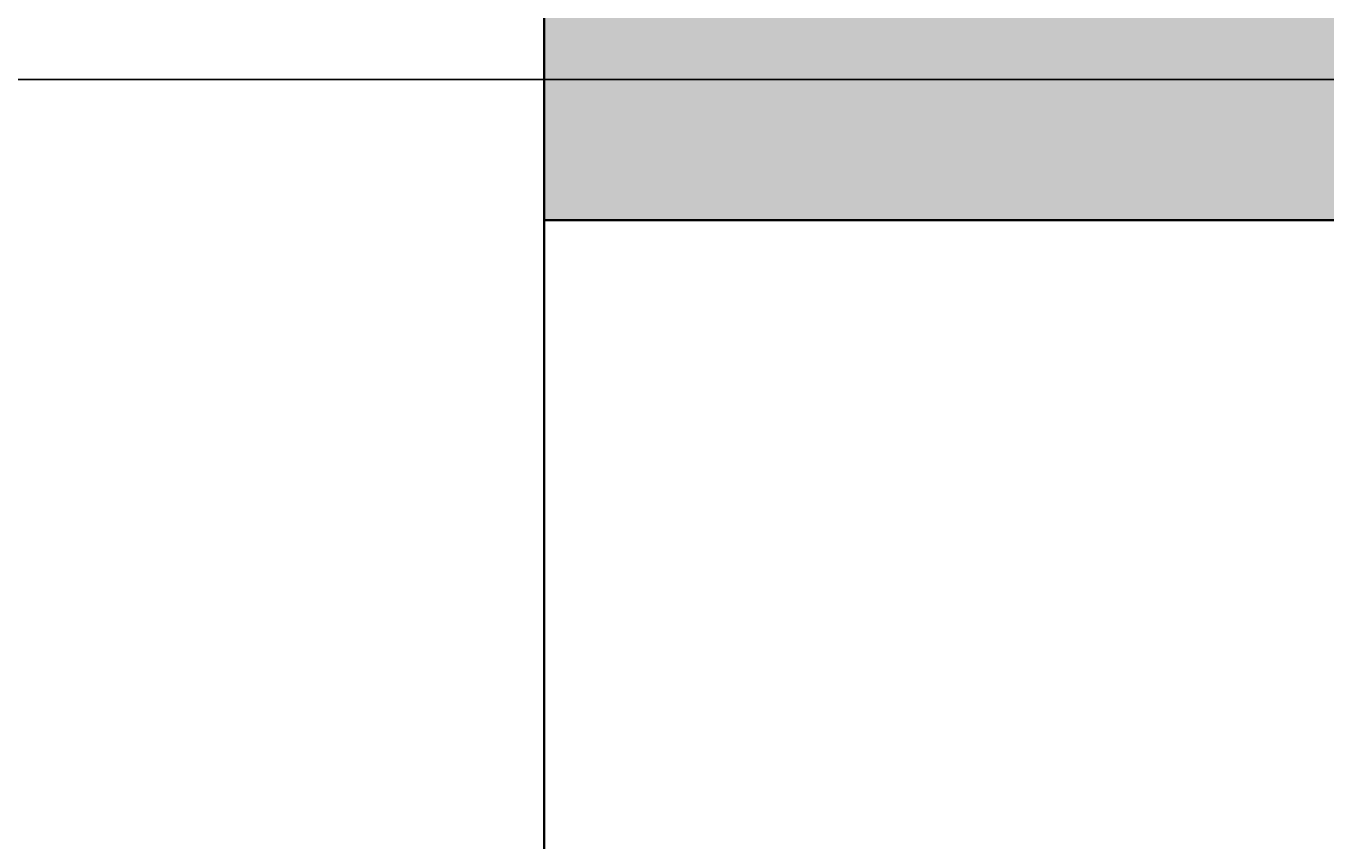
# Model space of a CAD drawing. Units: inches. Extents: x 1998 to 2588, y 1139 to 1977.
# Tile 102 of 134: x 2397 to 2425, y 1573 to 1590. Entities that reach past the tile are written whole.
import ezdxf

# ---------------------------------------------------------------- set-up
doc = ezdxf.new("R2010")
doc.units = ezdxf.units.IN
for name, color, linetype, lineweight in [('A-ANNO-DIMS', 2, 'Continuous', 18), ('A-FLOR-EVTR', 7, 'Continuous', 35), ('A-FLOR-STRS', 7, 'Continuous', 25), ('A-WALL-PATT', 252, 'Continuous', 13)]:
    doc.layers.add(name, color=color, linetype=linetype, lineweight=lineweight)
doc.styles.get("Standard").update_dxf_attribs({"font": 'arial.ttf'})
doc.dimstyles.get("Standard").update_dxf_attribs({"dimtxt": 0.18, "dimasz": 0.18, "dimexe": 0.18, "dimexo": 0.0625, "dimgap": 0.09, "dimtad": 0, "dimtih": 1, "dimtoh": 1, "dimdec": 4, "dimzin": 0, "dimdsep": 46, "dimtxsty": 'Standard', "dimcen": 0.09, "dimadec": 0, "dimazin": 0, "dimtfac": 1, "dimtdec": 4, "dimtofl": 0, "dimtmove": 0, "dimatfit": 3, "dimfxl": 1, "dimtolj": 1, "dimtzin": 0, "dimarcsym": 0})

# ---------------------------------------------------------------- blocks, each defined once
blk = doc.blocks.new('*D24')
at = {"layer": 'A-ANNO-DIMS', "color": 0, "lineweight": -2, "transparency": 16777216}
for p, q in [((2398.535, 1911.232), (2588.309, 1911.232)), ((2588.129, 1911.052), (2588.129, 1570.164)), ((2588.129, 1228.912), (2588.129, 1569.8)), ((2527.535, 1228.732), (2588.309, 1228.732))]:
    blk.add_line(p, q, dxfattribs=at)
at = {"layer": 'A-ANNO-DIMS', "color": 0, "transparency": 16777216}
for points in [[(2588.099, 1911.052), (2588.159, 1911.052), (2588.129, 1911.232)], [(2588.099, 1228.912), (2588.159, 1228.912), (2588.129, 1228.732)]]:
    blk.add_solid(points, dxfattribs=at)
at = {"layer": 'Defpoints', "color": 0, "transparency": 16777216}
for p in [(2398.473, 1911.232), (2588.129, 1911.232), (2527.473, 1228.732)]:
    blk.add_point(p, dxfattribs=at)
at = {"layer": 'A-ANNO-DIMS', "color": 0, "transparency": 16777216, "insert": (2588.129, 1569.982), "char_height": 0.18, "attachment_point": 5}
blk.add_mtext('\\A1;682.5', dxfattribs=at)
blk = doc.blocks.new('*D34')
at = {"layer": 'A-ANNO-DIMS', "color": 0, "lineweight": -2, "transparency": 16777216}
for p, q in [((2407.91, 1594.732), (1997.843, 1594.732)), ((1998.023, 1594.552), (1998.023, 1558.913)), ((1998.023, 1522.912), (1998.023, 1558.552)), ((2407.91, 1522.732), (1997.843, 1522.732))]:
    blk.add_line(p, q, dxfattribs=at)
at = {"layer": 'A-ANNO-DIMS', "color": 0, "transparency": 16777216}
for points in [[(1997.993, 1594.552), (1998.053, 1594.552), (1998.023, 1594.732)], [(1997.993, 1522.912), (1998.053, 1522.912), (1998.023, 1522.732)]]:
    blk.add_solid(points, dxfattribs=at)
at = {"layer": 'Defpoints', "color": 0, "transparency": 16777216}
for p in [(1998.023, 1594.732), (2407.973, 1594.732), (2407.973, 1522.732)]:
    blk.add_point(p, dxfattribs=at)
at = {"layer": 'A-ANNO-DIMS', "color": 0, "transparency": 16777216, "insert": (1998.023, 1558.732), "char_height": 0.18, "attachment_point": 5}
blk.add_mtext('\\A1;72', dxfattribs=at)
blk = doc.blocks.new('*D42')
at = {"layer": 'A-ANNO-DIMS', "color": 0, "lineweight": -2, "transparency": 16777216}
for p, q in [((2287.535, 1588.732), (2588.309, 1588.732)), ((2588.129, 1588.552), (2588.129, 1555.914)), ((2588.129, 1522.912), (2588.129, 1555.55)), ((2287.535, 1522.732), (2588.309, 1522.732))]:
    blk.add_line(p, q, dxfattribs=at)
at = {"layer": 'A-ANNO-DIMS', "color": 0, "transparency": 16777216}
for points in [[(2588.099, 1588.552), (2588.159, 1588.552), (2588.129, 1588.732)], [(2588.099, 1522.912), (2588.159, 1522.912), (2588.129, 1522.732)]]:
    blk.add_solid(points, dxfattribs=at)
at = {"layer": 'Defpoints', "color": 0, "transparency": 16777216}
for p in [(2287.473, 1588.732), (2588.129, 1588.732), (2287.473, 1522.732)]:
    blk.add_point(p, dxfattribs=at)
at = {"layer": 'A-ANNO-DIMS', "color": 0, "transparency": 16777216, "insert": (2588.129, 1555.732), "char_height": 0.18, "attachment_point": 5}
blk.add_mtext('\\A1;66', dxfattribs=at)
blk = doc.blocks.new('*D43')
at = {"layer": 'A-ANNO-DIMS', "color": 0, "lineweight": -2, "transparency": 16777216}
for p, q in [((2407.973, 1594.67), (2407.973, 1138.602)), ((2345.973, 1588.67), (2345.973, 1138.602)), ((2346.153, 1138.782), (2376.754, 1138.782)), ((2407.793, 1138.782), (2377.191, 1138.782))]:
    blk.add_line(p, q, dxfattribs=at)
at = {"layer": 'A-ANNO-DIMS', "color": 0, "transparency": 16777216}
for points in [[(2346.153, 1138.812), (2346.153, 1138.752), (2345.973, 1138.782)], [(2407.793, 1138.812), (2407.793, 1138.752), (2407.973, 1138.782)]]:
    blk.add_solid(points, dxfattribs=at)
at = {"layer": 'Defpoints', "color": 0, "transparency": 16777216}
for p in [(2407.973, 1594.732), (2345.973, 1588.732), (2407.973, 1138.782)]:
    blk.add_point(p, dxfattribs=at)
at = {"layer": 'A-ANNO-DIMS', "color": 0, "transparency": 16777216, "insert": (2376.973, 1138.782), "char_height": 0.18, "attachment_point": 5}
blk.add_mtext('\\A1;62', dxfattribs=at)

msp = doc.modelspace()

# ---------------------------------------------------------------- hatches: boundary and pattern name
at = {"layer": 'A-WALL-PATT'}
h = msp.add_hatch(color=256, dxfattribs=at)
h.dxf.hatch_style = 1
h.paths.add_polyline_path([(2527.4729, 1362.2324), (2510.9729, 1362.2324), (2510.9729, 1357.7324), (2518.4729, 1357.7324), (2518.4729, 1237.7324), (2503.1458, 1237.7324), (2503.1458, 1228.7324), (2527.4729, 1228.7324)])
h.paths.add_polyline_path([(2490.5682, 1362.2324), (2398.4729, 1362.2324), (2398.4729, 1357.7324), (2490.5682, 1357.7324)])
h.paths.add_polyline_path([(2224.9729, 1264.7324), (2222.9729, 1264.7324), (2222.9729, 1232.4125), (2341.4729, 1232.4125), (2341.4729, 1234.4125), (2224.9729, 1234.4125)])
h.paths.add_polyline_path([(2334.5332, 1273.7324), (2264.7638, 1273.7324), (2264.7638, 1269.5611, -0.043659), (2264.3413, 1264.7324), (2334.5332, 1264.7324)])
h.paths.add_polyline_path([(2236.9551, 1273.7324), (2234.4125, 1273.7324), (2234.4125, 1264.7324), (2236.9551, 1264.7324), (2236.9551, 1269.5611)])
h.paths.add_polyline_path([(2222.9729, 1293.2324), (2096.9729, 1293.2324), (2096.9729, 1345.0966), (2087.9729, 1345.0966), (2087.9729, 1284.2324), (2222.9729, 1284.2324), (2222.9729, 1285.137)])
h.paths.add_polyline_path([(2096.9729, 1458.7927), (2087.9729, 1458.7927), (2087.9729, 1417.7324), (2087.9729, 1413.2324), (2096.9729, 1413.2324), (2096.9729, 1417.7324)])
h.paths.add_polyline_path([(2096.9729, 1413.2324), (2087.9729, 1413.2324), (2087.9729, 1365.5012), (2096.9729, 1365.5012), (2096.9729, 1369.3358)])
h.paths.add_polyline_path([(2186.2943, 1417.7324), (2138.6074, 1417.7324), (2096.9729, 1417.7324), (2096.9729, 1413.2324), (2138.6074, 1413.2324), (2186.2943, 1413.2324)])
h.paths.add_polyline_path([(2181.4729, 1465.7324), (2176.9729, 1465.7324), (2176.9729, 1451.6434), (2181.4729, 1451.6434)])
h.paths.add_polyline_path([(2181.4729, 1422.1664), (2176.9729, 1422.1664), (2176.9729, 1417.7324), (2181.4729, 1417.7324)])
h.paths.add_polyline_path([(2063.9729, 1465.7324), (2087.9729, 1465.7324), (2087.9729, 1470.2324), (2059.4729, 1470.2324), (2059.4729, 1413.2324), (2087.9729, 1413.2324), (2087.9729, 1417.7324), (2063.9729, 1417.7324)])
h.paths.add_polyline_path([(2181.4729, 1755.2324), (2176.9729, 1755.2324), (2176.9729, 1748.6798), (2177.0513, 1748.6798), (2181.4729, 1748.6798)])
h.paths.add_polyline_path([(2227.4729, 1707.2324), (2220.4647, 1707.2324), (2220.4647, 1702.7324), (2222.9729, 1702.7324), (2222.9729, 1604.637), (2227.4729, 1604.637)])
h.paths.add_polyline_path([(2114.9729, 1702.7324), (2105.9729, 1702.7324), (2105.9729, 1628.4781, -0.0318759), (2110.1012, 1628.7416), (2114.9729, 1628.7416)])
h.paths.add_polyline_path([(2345.9729, 1739.3278), (2341.4729, 1739.3278), (2341.4729, 1647.5211), (2345.9729, 1647.5211)])
h.paths.add_polyline_path([(2350.6273, 1641.2324), (2345.9729, 1641.2324), (2345.9729, 1636.7324), (2350.6273, 1636.7324), (2350.6273, 1639.8729)])
h.paths.add_polyline_path([(2501.9729, 1641.2324), (2407.9729, 1641.2324), (2392.5005, 1641.2324), (2392.5005, 1639.8729), (2392.5005, 1636.7324), (2501.9729, 1636.7324)])
h.paths.add_polyline_path([(2510.9729, 1755.2324), (2501.9729, 1755.2324), (2501.9729, 1641.2324), (2510.9729, 1641.2324)])
h.paths.add_polyline_path([(2549.1786, 1641.2324), (2522.3775, 1641.2324), (2522.3775, 1636.7324), (2540.1786, 1636.7324), (2540.1786, 1480.7324), (2522.3775, 1480.7324), (2522.3775, 1476.2324), (2549.1786, 1476.2324)])
h.paths.add_polyline_path([(2498.1786, 1594.7324), (2407.9729, 1594.7324), (2407.9729, 1585.7324), (2416.9729, 1585.7324), (2489.1786, 1585.7324), (2489.1786, 1531.7324), (2416.9729, 1531.7324), (2407.9729, 1531.7324), (2407.9729, 1522.7324), (2498.1786, 1522.7324)])
h.paths.add_polyline_path([(2351.6437, 1480.7324), (2345.9729, 1480.7324), (2345.9729, 1476.2324), (2351.6437, 1476.2324), (2351.6437, 1477.5919)])
h.paths.add_polyline_path([(2501.9729, 1480.7324), (2498.1786, 1480.7324), (2407.9729, 1480.7324), (2393.5168, 1480.7324), (2393.5168, 1477.5919), (2393.5168, 1476.2324), (2501.9729, 1476.2324)])

# ---------------------------------------------------------------- linework, layer by layer
at = {"layer": 'A-FLOR-EVTR'}
msp.add_line((2416.9729, 1585.7324), (2407.9729, 1585.7324), dxfattribs=at)
msp.add_lwpolyline([(2407.9729, 1522.7324), (2498.1786, 1522.7324), (2498.1786, 1594.7324), (2407.9729, 1594.7324)], close=True, dxfattribs=at)
msp.add_lwpolyline([(2416.9729, 1531.7324), (2489.1786, 1531.7324), (2489.1786, 1585.7324), (2416.9729, 1585.7324)], dxfattribs=at)
at = {"layer": 'A-FLOR-STRS'}
msp.add_line((2407.9729, 1480.7324), (2407.9729, 1636.7324), dxfattribs=at)

# ---------------------------------------------------------------- dimensions: what is measured, and where the dimension line sits
at = {"layer": 'A-ANNO-DIMS'}
for base, p1, p2, override, picture, middle in [((2588.1286, 1911.2324), (2527.4729, 1228.7324), (2398.4729, 1911.2324), {"dimdec": 1, "dimlfac": 1, "dimrnd": 0, "dimzin": 0, "dimdsep": 46, "dimlunit": 2}, '*D24', (2588.1286, 1569.9824)), ((1998.0229, 1594.7324), (2407.9729, 1522.7324), (2407.9729, 1594.7324), {"dimdec": 0, "dimlfac": 1, "dimrnd": 0, "dimzin": 0, "dimdsep": 46, "dimlunit": 2}, '*D34', (1998.0229, 1558.7324)), ((2588.1286, 1588.7324), (2287.4729, 1522.7324), (2287.4729, 1588.7324), {"dimdec": 0, "dimlfac": 1, "dimrnd": 0, "dimzin": 0, "dimdsep": 46, "dimlunit": 2}, '*D42', (2588.1286, 1555.7324))]:
    dim = msp.add_linear_dim(base=base, p1=p1, p2=p2, angle=90, dimstyle='Standard', override=override, dxfattribs=at)
    dim.commit()
    dim.dimension.update_dxf_attribs({"geometry": picture, "text_midpoint": middle})
dim = msp.add_linear_dim(base=(2407.9729, 1138.7824), p1=(2345.9729, 1588.7324), p2=(2407.9729, 1594.7324), dimstyle='Standard', override={"dimdec": 0, "dimlfac": 1, "dimrnd": 0, "dimzin": 0, "dimdsep": 46, "dimlunit": 2}, dxfattribs=at)
dim.commit()
dim.dimension.update_dxf_attribs({"geometry": '*D43', "text_midpoint": (2376.9729, 1138.7824)})

doc.saveas('drawing.dxf')
